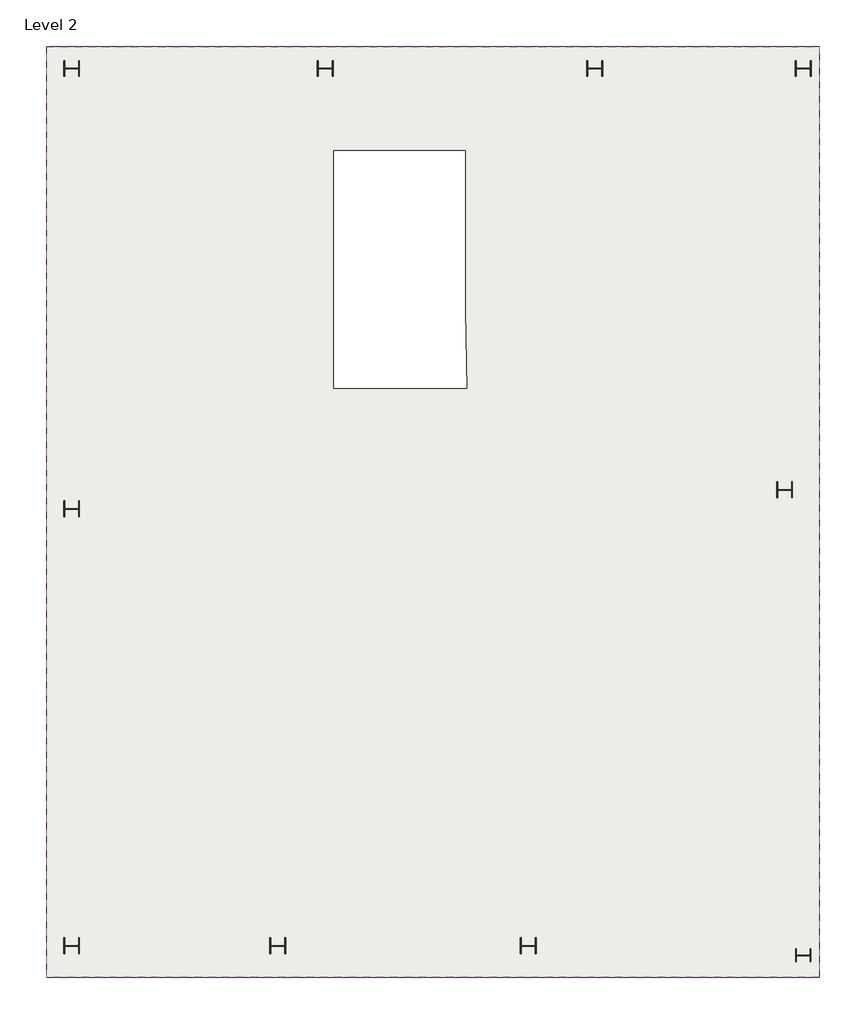
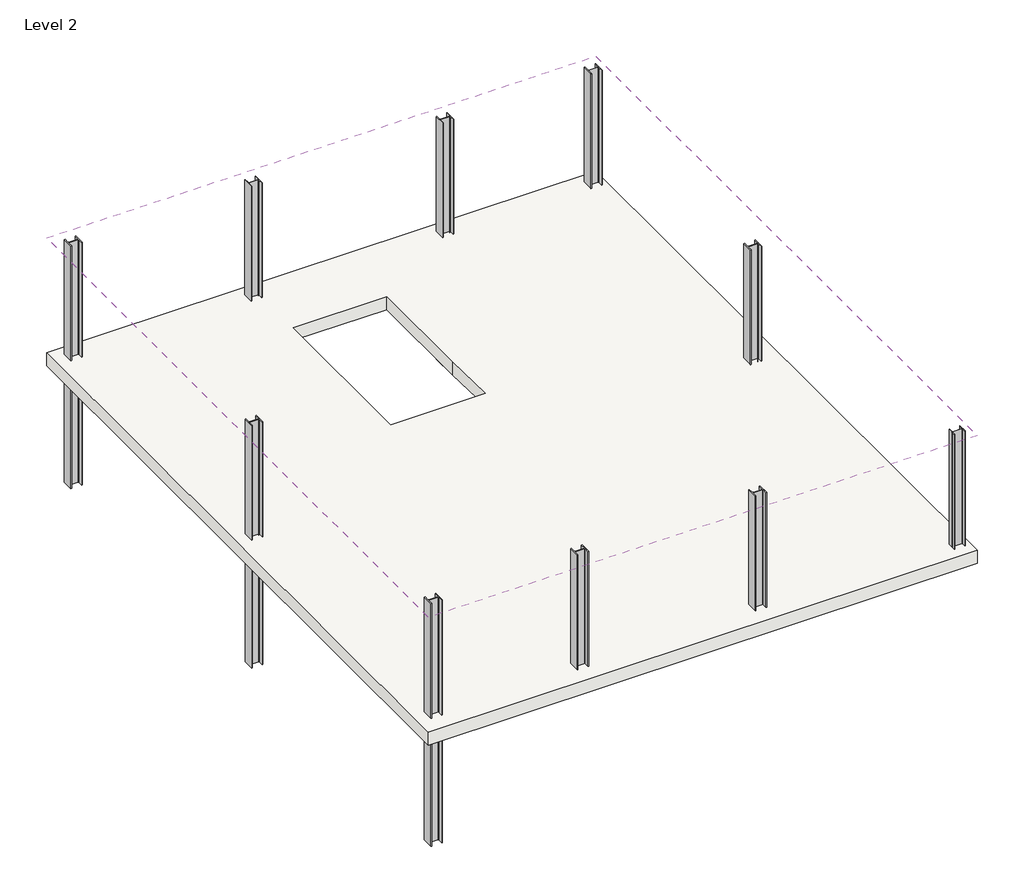
# One storey: 10 columns, 2 roofs.
"""IFC4 building model written with IfcOpenShell, lengths in millimetres."""

from ifc_helpers import new_model, si_unit, frame, origin, place, context, project, spatial, polyline, outline, extrude, transform, mapped, element, save
from components import w_shapes_column_w10x33_9bdcd76c, w_shapes_column_w10x49_ceff5d29, w_shapes_column_w10x49_2dae7ecb

model = new_model("IFC4")

# Units and contexts
model_context = context("Model", 3, world=origin())
ifc_project = project(units=[si_unit("LENGTHUNIT", "METRE", prefix="MILLI")], contexts=[model_context])

# Site, building, storey
site = spatial("IfcSite", under=ifc_project)
building = spatial("IfcBuilding", under=site)
storey = spatial("IfcBuildingStorey", under=building, Name="Level 2", Elevation=3048.0)

# Columns
placement = place(None, origin())
w_shapes_column_w10x33_shape = w_shapes_column_w10x33_9bdcd76c(model_context)
element("IfcColumn", 1, ObjectType="W Shapes-Column : W10X33", at=placement, inside=storey, context=model_context, shape_type="MappedRepresentation", body=[
    mapped(w_shapes_column_w10x33_shape, transform((9567.7250253, -6216.5472691, 0.0), x_axis=(0.0, 1.0000000000000002, 0.0), y_axis=(-1.0000000000000002, 0.0, 0.0), z_axis=(0.0, 0.0, 1.0))),
])
w_shapes_column_w10x49_shape = w_shapes_column_w10x49_ceff5d29(model_context)
element("IfcColumn", 2, ObjectType="W Shapes-Column : W10X49", at=placement, inside=storey, context=model_context, shape_type="MappedRepresentation", body=[
    mapped(w_shapes_column_w10x49_shape, transform((1134.9250253, -6064.1472691, 0.0), x_axis=(0.0, 1.0000000000000002, 0.0), y_axis=(-1.0000000000000002, 0.0, 0.0), z_axis=(0.0, 0.0, 1.0))),
])
element("IfcColumn", 3, ObjectType="W Shapes-Column : W10X49", at=placement, inside=storey, context=model_context, shape_type="MappedRepresentation", body=[
    mapped(w_shapes_column_w10x49_shape, transform((5152.9635307, -6064.1472691, 0.0), x_axis=(0.0, 1.0000000000000002, 0.0), y_axis=(-1.0000000000000002, 0.0, 0.0), z_axis=(0.0, 0.0, 1.0))),
])
w_shapes_column_w10x49_2_shape = w_shapes_column_w10x49_2dae7ecb(model_context)
element("IfcColumn", 4, ObjectType="W Shapes-Column : W10X49", at=placement, inside=storey, context=model_context, shape_type="MappedRepresentation", body=[
    mapped(w_shapes_column_w10x49_2_shape, transform((-2171.8374747, 8012.2152309, 0.0), x_axis=(0.0, 1.0000000000000002, 0.0), y_axis=(-1.0000000000000002, 0.0, 0.0), z_axis=(0.0, 0.0, 1.0))),
])
element("IfcColumn", 5, ObjectType="W Shapes-Column : W10X49", at=placement, inside=storey, context=model_context, shape_type="MappedRepresentation", body=[
    mapped(w_shapes_column_w10x49_2_shape, transform((1896.9250253, 8012.2152309, 0.0), x_axis=(0.0, 1.0000000000000002, 0.0), y_axis=(-1.0000000000000002, 0.0, 0.0), z_axis=(0.0, 0.0, 1.0))),
])
element("IfcColumn", 6, ObjectType="W Shapes-Column : W10X49", at=placement, inside=storey, context=model_context, shape_type="MappedRepresentation", body=[
    mapped(w_shapes_column_w10x49_2_shape, transform((6219.6875253, 8012.2152309, 0.0), x_axis=(0.0, 1.0000000000000002, 0.0), y_axis=(-1.0000000000000002, 0.0, 0.0), z_axis=(0.0, 0.0, 1.0))),
])
element("IfcColumn", 7, ObjectType="W Shapes-Column : W10X49", at=placement, inside=storey, context=model_context, shape_type="MappedRepresentation", body=[
    mapped(w_shapes_column_w10x49_2_shape, transform((9567.7250253, 8012.2152309, 0.0), x_axis=(0.0, 1.0000000000000002, 0.0), y_axis=(-1.0000000000000002, 0.0, 0.0), z_axis=(0.0, 0.0, 1.0))),
])
element("IfcColumn", 8, ObjectType="W Shapes-Column : W10X49", at=placement, inside=storey, context=model_context, shape_type="MappedRepresentation", body=[
    mapped(w_shapes_column_w10x49_2_shape, transform((-2171.8374747, -6064.1472691, 0.0), x_axis=(0.0, 1.0000000000000002, 0.0), y_axis=(-1.0000000000000002, 0.0, 0.0), z_axis=(0.0, 0.0, 1.0))),
])
element("IfcColumn", 9, ObjectType="W Shapes-Column : W10X49", at=placement, inside=storey, context=model_context, shape_type="MappedRepresentation", body=[
    mapped(w_shapes_column_w10x49_2_shape, transform((-2171.8374747, 946.2527309, 0.0), x_axis=(0.0, 1.0000000000000002, 0.0), y_axis=(-1.0000000000000002, 0.0, 0.0), z_axis=(0.0, 0.0, 1.0))),
])
element("IfcColumn", 10, ObjectType="W Shapes-Column : W10X49", at=placement, inside=storey, context=model_context, shape_type="MappedRepresentation", body=[
    mapped(w_shapes_column_w10x49_2_shape, transform((9267.6875253, 1251.0527309, 0.0), x_axis=(0.0, 1.0000000000000002, 0.0), y_axis=(-1.0000000000000002, 0.0, 0.0), z_axis=(0.0, 0.0, 1.0))),
])

# Roofs
element("IfcRoof", 11, ObjectType="Generic - 12\"", at=placement, inside=storey, context=model_context, shape_type="SweptSolid", body=[
    extrude(outline(polyline([(-2573.4749747, 8363.0527309), (9821.7250253, 8363.0527309), (9821.7250253, -6572.1472691), (-2573.4749747, -6572.1472691), (-2573.4749747, 8363.0527309)]), holes=[polyline([(4142.2535874, 4128.9601827), (4142.2535874, 6691.9427876), (2034.0535874, 6691.9427876), (2034.0535874, 2881.9427876), (4167.6535874, 2881.9427876), (4142.2535874, 4128.9601827)])]), frame((0.0, 0.0, 3048.0), z_axis=(0.0, 0.0, 1.0), x_axis=(1.0, 0.0, 0.0)), (0.0, 0.0, 1.0), 304.8),
])
element("IfcRoof", 12, ObjectType="Generic - 9\"", at=placement, inside=storey, context=model_context, shape_type="SweptSolid", body=[
    extrude(outline(polyline([(-2573.4749747, 8363.0527309), (9821.7250253, 8363.0527309), (9821.7250253, -6572.1472691), (-2573.4749747, -6572.1472691), (-2573.4749747, 8363.0527309)])), frame((0.0, 0.0, 6096.0), z_axis=(0.0, 0.0, 1.0), x_axis=(1.0, 0.0, 0.0)), (0.0, 0.0, 1.0), 228.6),
])

save(model, "model.ifc")

# Revit data of these elements
# Type "W Shapes-Column : W10X33"
#   Section Name Key = "W10x33"
#   Assembly Code = "B10"
#   Width = 7.960"
#   Web Thickness = 0.290"
#   Web Fillet = 0.500"
#   Warping Constant = 791.00 in⁶
#   Torsional Moment of Inertia = 0.583 in⁴
#   Section Area = 9.71 in²
#   Plastic Modulus weak axis = 14.00 in³
#   Plastic Modulus strong axis = 38.80 in³
#   Perimeter = 49.90 ft²/ft
#   Nominal Weight = 33.00 lbf/ft
#   Moment of Inertia weak axis = 36.60 in⁴
#   Moment of Inertia strong axis = 171.00 in⁴
#   Height = 9.730"
#   Flange Thickness = 0.440"
#   Elastic Modulus weak axis = 9.20 in³
#   Elastic Modulus strong axis = 35.00 in³
#   Centroid Vertical = 4.865"
#   Centroid Horizontal = 3.980"
#   Structural Material [instance default] = Steel ASTM A992
#   Principal Axes Angle = 0
# Type "W Shapes-Column : W10X49"
#   Section Name Key = "W10x49"
#   Assembly Code = "B10"
#   Width = 10.000"
#   Web Thickness = 0.340"
#   Web Fillet = 0.500"
#   Warping Constant = 2070.00 in⁶
#   Torsional Moment of Inertia = 1.39 in⁴
#   Section Area = 14.40 in²
#   Plastic Modulus weak axis = 28.30 in³
#   Plastic Modulus strong axis = 60.40 in³
#   Perimeter = 58.50 ft²/ft
#   Nominal Weight = 49.00 lbf/ft
#   Moment of Inertia weak axis = 93.40 in⁴
#   Moment of Inertia strong axis = 272.00 in⁴
#   Height = 10.000"
#   Flange Thickness = 0.560"
#   Elastic Modulus weak axis = 18.70 in³
#   Elastic Modulus strong axis = 54.60 in³
#   Centroid Vertical = 5.000"
#   Centroid Horizontal = 5.000"
#   Structural Material [instance default] = Steel ASTM A992
#   Principal Axes Angle = 0
# Type "Generic - 12\""
#   Assembly Code = "B1020"
#   Layers, outside or top first: 1' - 0" no material (function 1)
# Type "Generic - 9\""
#   Assembly Code = "B1020"
#   Layers, outside or top first: 0' - 9" no material (function 1)
# Element 1 (IfcColumn, "W Shapes-Column : W10X33")
#   Structural Material = Steel ASTM A992
#   Phase Created = New Construction
#   Materials on its faces: "Steel ASTM A992"
# Elements 2, 3, 4, 5, 6, 7, 8, 9, 10 (IfcColumn, "W Shapes-Column : W10X49")
#   Structural Material = Steel ASTM A992
#   Phase Created = New Construction
#   Materials on its faces: "Steel ASTM A992"
# Element 11 (IfcRoof, "Generic - 12\"")
#   built-in parameter 1001705 = 11 (stored number, unit not read)
#   built-in parameter 1001710 = 33615
#   Phase Created = New Construction
#   Materials on its faces: "Default Roof"
# Element 12 (IfcRoof, "Generic - 9\"")
#   built-in parameter 1001705 = 20.75 (stored number, unit not read)
#   built-in parameter 1001701 = 10 (stored number, unit not read)
#   built-in parameter 1001710 = 33615
#   Phase Created = New Construction
#   Materials on its faces: "Default Roof"
# Materials
#   "Steel ASTM A992": class "Metal", colour RGB 199 199 199, transparency 0, Description = "Structural steel 50ksi", Cost = 0
#   "Default Roof": colour RGB 88 101 114, transparency 0
